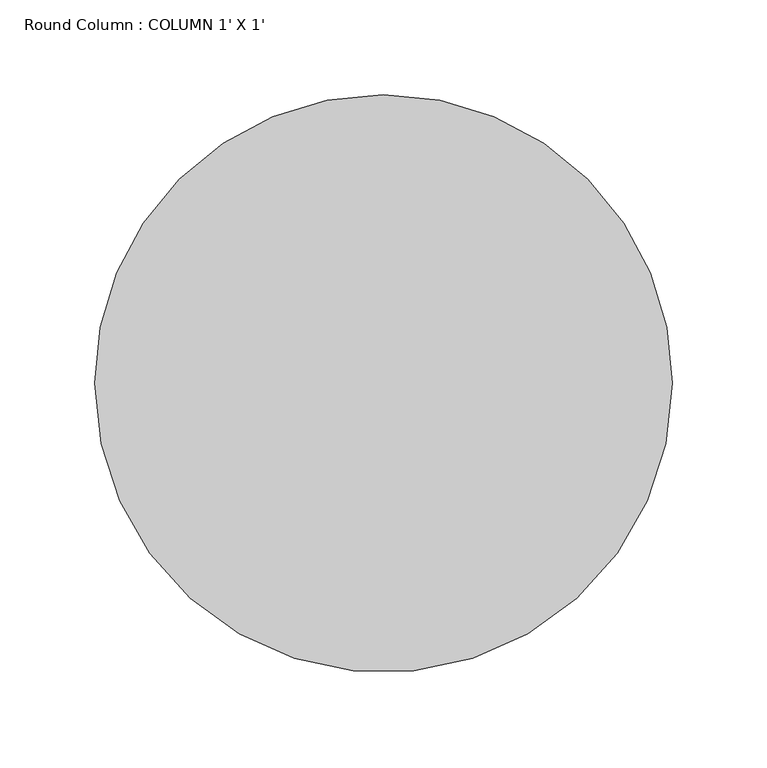
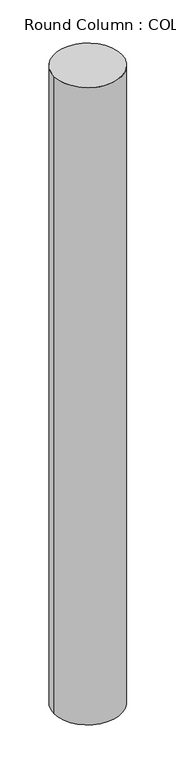
"""IFC4 building model written with IfcOpenShell, lengths in millimetres: column geometry, Round Column : COLUMN 1' X 1'."""

from ifc_helpers import new_model, si_unit, point, frame, origin, origin_2d, place, context, project, spatial, circle_curve, trimmed, segment, composite_curve, outline, extrude, source, transform, mapped, element, save


def round_column_column_1_x_1_3d9dadd9(model_context):
    return source(origin(), model_context, "Body", "SweptSolid", [
        extrude(outline(composite_curve([segment(trimmed(circle_curve(origin_2d(), 152.4), [point((152.4, 0.0))], [point((-152.4, 0.0))], False, "CARTESIAN"), True, "CONTINUOUS"), segment(trimmed(circle_curve(origin_2d(), 152.4), [point((-152.4, 0.0))], [point((0.0, 152.4))], False, "CARTESIAN"), True, "CONTINUOUS"), segment(trimmed(circle_curve(origin_2d(), 152.4), [point((0.0, 152.4))], [point((152.4, 0.0))], False, "CARTESIAN"), True, "CONTINUOUS")], self_intersect=False)), frame((0.0, 0.0, 304.8), z_axis=(0.0, 0.0, 1.0), x_axis=(1.0, 0.0, 0.0)), (0.0, 0.0, 1.0), 3048.0),
    ])


if __name__ == "__main__":
    model = new_model("IFC4")
    model_context = context("Model", 3, world=origin())
    ifc_project = project(units=[si_unit("LENGTHUNIT", "METRE", prefix="MILLI")], contexts=[model_context])
    site = spatial("IfcSite", under=ifc_project)
    building = spatial("IfcBuilding", under=site)
    placement = place(None, origin())
    round_column_column_1_x_1_shape = round_column_column_1_x_1_3d9dadd9(model_context)
    element("IfcColumn", 1, ObjectType="Round Column : COLUMN 1' X 1'", at=placement, inside=building, context=model_context, shape_type="MappedRepresentation", body=[
        mapped(round_column_column_1_x_1_shape, transform((0.0, 0.0, 0.0), x_axis=(1.0, 0.0, 0.0), y_axis=(0.0, 1.0, 0.0), z_axis=(0.0, 0.0, 1.0))),
    ])
    save(model, "model.ifc")

# Revit data of these elements
# Type "Round Column : COLUMN 1' X 1'"
#   Assembly Code = "B1010200"
#   Diameter = 1' - 0"
#   Offset Base = 0' - 0"
#   Offset Top = 0' - 0"
#   Material = CREAM BEIGE COLOUR
# Element 1 (IfcColumn, "Round Column : COLUMN 1' X 1'")
#   Materials on its faces: "CREAM BEIGE COLOUR"
# Materials
#   "CREAM BEIGE COLOUR": class "Generic", colour RGB 120 120 120, transparency 0, Cost = 0
